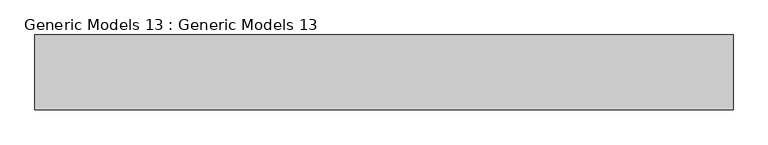
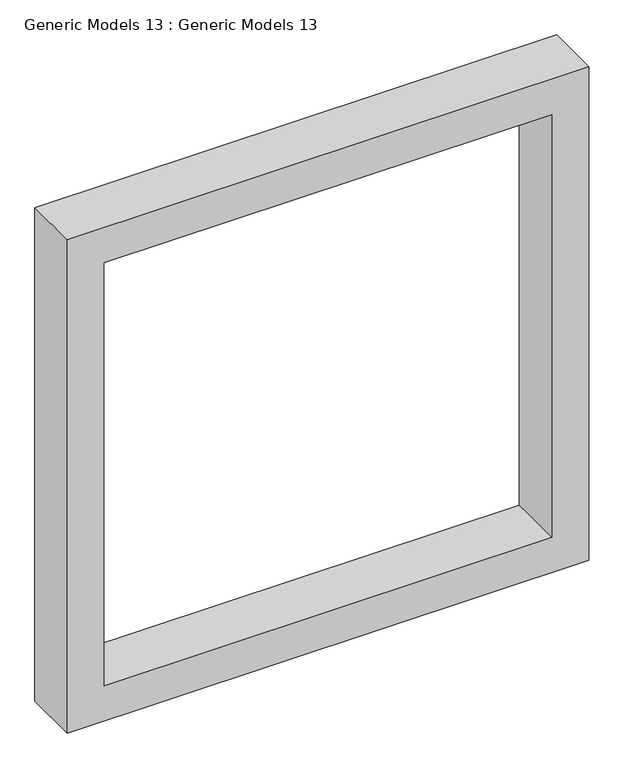
"""IFC4 building model written with IfcOpenShell, lengths in millimetres: proxy geometry, Generic Models 13 : Generic Models 13."""

from ifc_helpers import new_model, si_unit, frame, origin, place, context, project, spatial, polyline, outline, extrude, source, transform, mapped, element, save


def generic_models_13_generic_models_13_6edbfaa0(model_context):
    return source(origin(), model_context, "Body", "SweptSolid", [
        extrude(outline(polyline([(11769.6, 3021.0824202), (10347.2, 3021.0824202), (10347.2, 4443.4824202), (11769.6, 4443.4824202), (11769.6, 3021.0824202)]), holes=[polyline([(11668.0, 3122.6824202), (11668.0, 4341.8824202), (10448.8, 4341.8824202), (10448.8, 3122.6824202), (11668.0, 3122.6824202)])]), frame((0.0, -1223.6061634, 0.0), z_axis=(0.0, 1.0, 0.0), x_axis=(0.0, 0.0, 1.0)), (0.0, 0.0, 1.0), 152.4),
    ])


if __name__ == "__main__":
    model = new_model("IFC4")
    model_context = context("Model", 3, world=origin())
    ifc_project = project(units=[si_unit("LENGTHUNIT", "METRE", prefix="MILLI")], contexts=[model_context])
    site = spatial("IfcSite", under=ifc_project)
    building = spatial("IfcBuilding", under=site)
    placement = place(None, origin())
    generic_models_13_generic_models_13_shape = generic_models_13_generic_models_13_6edbfaa0(model_context)
    element("IfcBuildingElementProxy", 1, Name="Generic Models 13 : Generic Models 13", ObjectType="Generic Models 13 : Generic Models 13", at=placement, inside=building, context=model_context, shape_type="MappedRepresentation", body=[
        mapped(generic_models_13_generic_models_13_shape, transform((0.0, 0.0, 0.0), x_axis=(1.0, 0.0, 0.0), y_axis=(0.0, 1.0, 0.0), z_axis=(0.0, 0.0, 1.0))),
    ])
    save(model, "model.ifc")

# Revit data of these elements
# Element 1 (IfcBuildingElementProxy, "Generic Models 13 : Generic Models 13")
#   Materials on its faces: "black accent wall"
# Materials
#   "black accent wall": class "Generic", colour RGB 120 120 120, transparency 0, Cost = 0
